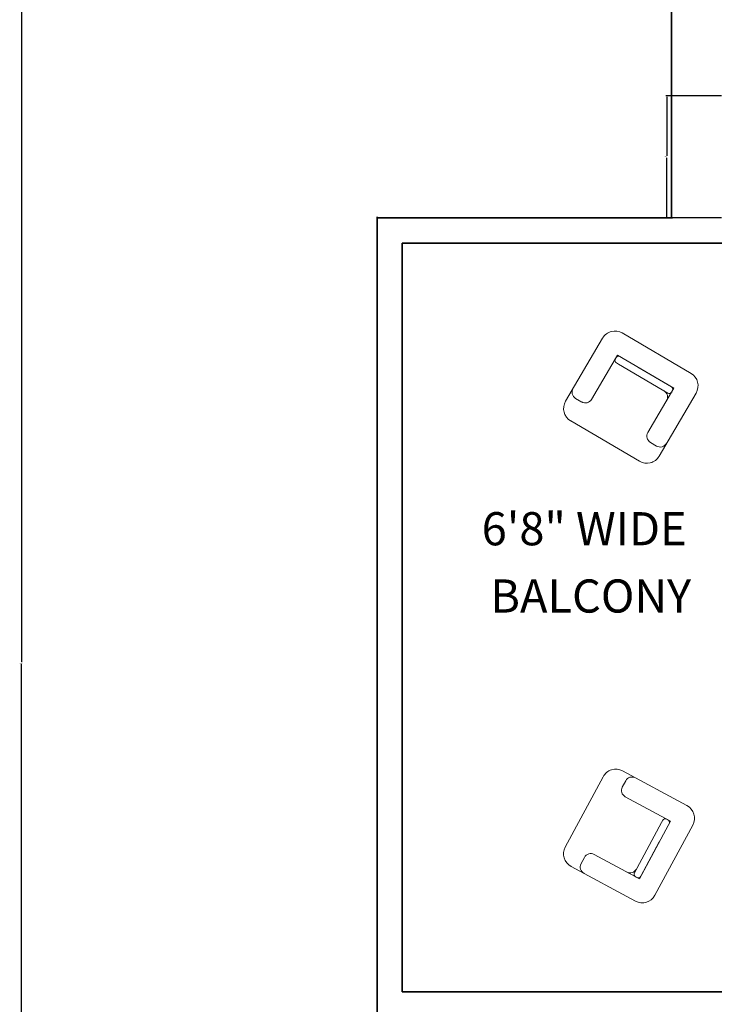
# Model space of a CAD drawing. Units: millimetres. Extents: x 27017497 to 27018854, y 7058029 to 7059154.
# Tile 31 of 91: x 27017497 to 27017621, y 7058297 to 7058472. Entities that reach past the tile are written whole.
import ezdxf

# ---------------------------------------------------------------- set-up
doc = ezdxf.new("R2010")
doc.units = ezdxf.units.MM
for name, color, linetype, lineweight in [('A-ANNO-DIMS', 2, 'Continuous', 18), ('A-AREA-IDEN', 7, 'Continuous', 18), ('A-FURN', 8, 'Continuous', 18), ('A-WALL', 7, 'Continuous', 35)]:
    doc.layers.add(name, color=color, linetype=linetype, lineweight=lineweight)
doc.styles.get("Standard").update_dxf_attribs({"font": 'arial.ttf'})
doc.dimstyles.get("Standard").update_dxf_attribs({"dimtxt": 0.18, "dimasz": 0.18, "dimexe": 0.18, "dimexo": 0.0625, "dimgap": 0.09, "dimtad": 0, "dimtih": 1, "dimtoh": 1, "dimdec": 4, "dimzin": 0, "dimdsep": 46, "dimtxsty": 'Standard', "dimcen": 0.09, "dimadec": 0, "dimazin": 0, "dimtfac": 1, "dimtdec": 4, "dimtofl": 0, "dimtmove": 0, "dimatfit": 3, "dimfxl": 1, "dimtolj": 1, "dimtzin": 0, "dimarcsym": 0})

# ---------------------------------------------------------------- blocks, each defined once
blk = doc.blocks.new('CHAIR-OCCASIONAL')
for p, q in [((19.6, 18.74), (7.02, 22.21)), ((3.87, 20.42), (0.09, 6.71)), ((4.13, 6.92), (7.23, 18.17)), ((5.25, 10.97), (7.23, 18.17)), ((5.25, 10.97), (7.1, 17.68)), ((16.06, 15.73), (7.23, 18.17)), ((7.23, 18.17), (16.06, 15.73)), ((7.23, 18.17), (16.06, 15.73)), ((7.73, 18.03), (7.97, 17.97)), ((7.73, 18.03), (7.97, 17.97)), ((17.64, 16.63), (17.98, 17.86)), ((17.64, 16.63), (17.98, 17.86)), ((8.33, 17.34), (5.63, 7.52)), ((17.6, 1.88), (21.39, 15.6)), ((5.63, 7.52), (5.5, 7.07)), ((12.96, 4.48), (4.13, 6.92)), ((4.87, 6.71), (4.63, 6.78)), ((1.88, 3.56), (14.46, 0.09)), ((13.86, 2.91), (13.52, 1.68))]:
    blk.add_line(p, q)
for centre, radius, start, end in [((6.34, 19.74), 2.56, 74.5879, 164.5879), ((16.74, 18.2), 1.28, 344.5879, 74.5879), ((16.74, 18.2), 1.28, 344.5879, 74.5879), ((7.59, 17.54), 0.512, 74.5879, 164.5879), ((7.84, 17.47), 0.512, 344.5879, 74.5879), ((18.92, 16.28), 2.56, 344.5879, 74.5879), ((9.36, 16.26), 1.28, 74.5879, 164.5879), ((16.4, 16.97), 1.28, 254.5879, 344.5879), ((16.4, 16.97), 1.28, 254.5879, 344.5879), ((4.76, 7.28), 0.512, 164.5879, 254.5879), ((5.01, 7.21), 0.512, 254.5879, 344.5879), ((2.56, 6.03), 2.56, 164.5879, 254.5879), ((12.62, 3.25), 1.28, 344.5879, 74.5879), ((15.14, 2.56), 2.56, 254.5879, 344.5879), ((12.28, 2.02), 1.28, 254.5879, 344.5879)]:
    blk.add_arc(centre, radius, start, end)
blk = doc.blocks.new('*D46')
at = {"layer": 'A-ANNO-DIMS', "color": 0, "lineweight": -2, "transparency": 16777216}
for p, q in [((27017622.6, 7058458.64), (27017612.7, 7058458.64)), ((27017612.88, 7058458.46), (27017612.88, 7058447.95)), ((27017612.88, 7058437.08), (27017612.88, 7058447.59)), ((27017622.6, 7058436.9), (27017612.7, 7058436.9))]:
    blk.add_line(p, q, dxfattribs=at)
at = {"layer": 'A-ANNO-DIMS', "color": 0, "transparency": 16777216}
for points in [[(27017612.85, 7058458.46), (27017612.91, 7058458.46), (27017612.88, 7058458.64)], [(27017612.85, 7058437.08), (27017612.91, 7058437.08), (27017612.88, 7058436.9)]]:
    blk.add_solid(points, dxfattribs=at)
at = {"layer": 'Defpoints', "color": 0, "transparency": 16777216}
for p in [(27017612.88, 7058458.64), (27017622.67, 7058458.64), (27017622.67, 7058436.9)]:
    blk.add_point(p, dxfattribs=at)
at = {"layer": 'A-ANNO-DIMS', "color": 0, "transparency": 16777216, "insert": (27017612.88, 7058447.77), "char_height": 0.18, "attachment_point": 5}
blk.add_mtext('\\A1;22 TYP.', dxfattribs=at)
blk = doc.blocks.new('*D48')
at = {"layer": 'A-ANNO-DIMS', "color": 0, "lineweight": -2, "transparency": 16777216}
for p, q in [((27018463.5, 7058622.91), (27017497.54, 7058622.91)), ((27017497.72, 7058622.73), (27017497.72, 7058357.75)), ((27017497.72, 7058092.41), (27017497.72, 7058357.39)), ((27018555.13, 7058092.23), (27017497.54, 7058092.23))]:
    blk.add_line(p, q, dxfattribs=at)
at = {"layer": 'A-ANNO-DIMS', "color": 0, "transparency": 16777216}
for points in [[(27017497.69, 7058622.73), (27017497.75, 7058622.73), (27017497.72, 7058622.91)], [(27017497.69, 7058092.41), (27017497.75, 7058092.41), (27017497.72, 7058092.23)]]:
    blk.add_solid(points, dxfattribs=at)
at = {"layer": 'Defpoints', "color": 0, "transparency": 16777216}
for p in [(27018463.56, 7058622.91), (27017497.72, 7058092.23), (27018555.19, 7058092.23)]:
    blk.add_point(p, dxfattribs=at)
at = {"layer": 'A-ANNO-DIMS', "color": 0, "transparency": 16777216, "insert": (27017497.72, 7058357.57), "char_height": 0.18, "attachment_point": 5}
blk.add_mtext('\\A1;530.7', dxfattribs=at)

msp = doc.modelspace()

# ---------------------------------------------------------------- linework, layer by layer
at = {"layer": 'A-WALL'}
for p, q in [((27017613.666, 7058589.912), (27017613.666, 7058437.098)), ((27017561.166, 7058437.098), (27017561.166, 7058294.412)), ((27017561.382, 7058436.905), (27017613.882, 7058436.905)), ((27017565.666, 7058432.412), (27017565.666, 7058298.912)), ((27017565.666, 7058432.412), (27017632.166, 7058432.412)), ((27017565.666, 7058298.912), (27017632.166, 7058298.912))]:
    msp.add_line(p, q, dxfattribs=at)

# ---------------------------------------------------------------- block references
at = {"layer": 'A-FURN'}
for p, rotation in [((27017598.452, 7058418.198), 254.9680663142556), ((27017619.069, 7058335.139), 167.1010863275715)]:
    msp.add_blockref('CHAIR-OCCASIONAL', p, dxfattribs=dict(at, rotation=rotation))

# ---------------------------------------------------------------- texts
at = {"layer": 'A-ANNO-DIMS'}
msp.add_text('6\'8" WIDE', height=5.9118, dxfattribs=at).set_placement((27017579.829, 7058378.509))
at = {"layer": 'A-AREA-IDEN'}
msp.add_text('BALCONY', height=5.9118, dxfattribs=at).set_placement((27017581.364, 7058366.512))

# ---------------------------------------------------------------- dimensions: what is measured, and where the dimension line sits
at = {"layer": 'A-ANNO-DIMS'}
dim = msp.add_linear_dim(base=(27017497.716, 7058092.23), p1=(27018463.561, 7058622.912), p2=(27018555.192, 7058092.23), angle=90, dimstyle='Standard', override={"dimdec": 1, "dimlfac": 1, "dimrnd": 0, "dimzin": 0, "dimdsep": 46, "dimlunit": 2}, dxfattribs=at)
dim.commit()
dim.dimension.update_dxf_attribs({"geometry": '*D48', "text_midpoint": (27017497.716, 7058357.571)})
dim = msp.add_linear_dim(base=(27017612.883, 7058458.642), p1=(27017622.665, 7058436.905), p2=(27017622.665, 7058458.642), angle=90, text='<> TYP.', dimstyle='Standard', override={"dimdec": 0, "dimlfac": 1, "dimrnd": 0, "dimzin": 0, "dimdsep": 46, "dimlunit": 2}, dxfattribs=at)
dim.commit()
dim.dimension.update_dxf_attribs({"geometry": '*D46', "text_midpoint": (27017612.883, 7058447.773)})

doc.saveas('drawing.dxf')
